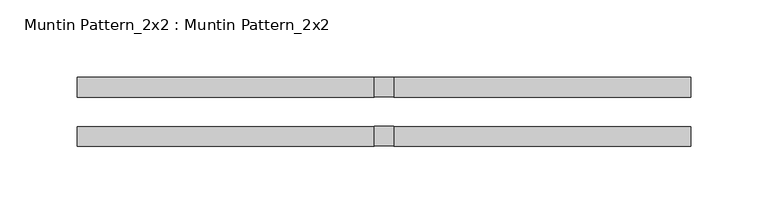
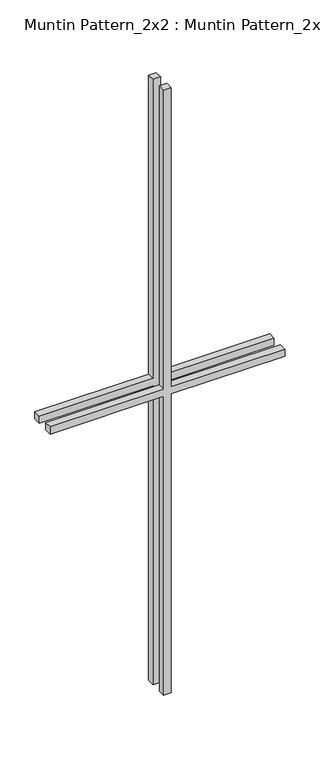
"""IFC4 building model written with IfcOpenShell, lengths in millimetres: proxy geometry, Muntin Pattern_2x2 : Muntin Pattern_2x2."""

from ifc_helpers import new_model, si_unit, frame, origin, place, context, project, spatial, polyline, outline, extrude, source, transform, mapped, element, save


def muntin_pattern_2x2_muntin_pattern_2x2_529c3de1(model_context):
    return source(origin(), model_context, "Body", "SweptSolid", [
        extrude(outline(polyline([(546.1, -6.35), (546.1, -198.4375), (533.4, -198.4375), (533.4, -6.35), (0.0, -6.35), (0.0, 6.35), (533.4, 6.35), (533.4, 198.4375), (546.1, 198.4375), (546.1, 6.35), (1079.5, 6.35), (1079.5, -6.35), (546.1, -6.35)])), frame((0.0, -22.225, 0.0), z_axis=(0.0, 1.0, 0.0), x_axis=(0.0, 0.0, 1.0)), (0.0, 0.0, 1.0), 12.7),
        extrude(outline(polyline([(546.1, -6.35), (546.1, -198.4375), (533.4, -198.4375), (533.4, -6.35), (0.0, -6.35), (0.0, 6.35), (533.4, 6.35), (533.4, 198.4375), (546.1, 198.4375), (546.1, 6.35), (1079.5, 6.35), (1079.5, -6.35), (546.1, -6.35)])), frame((0.0, 9.525, 0.0), z_axis=(0.0, 1.0, 0.0), x_axis=(0.0, 0.0, 1.0)), (0.0, 0.0, 1.0), 12.7),
    ])


if __name__ == "__main__":
    model = new_model("IFC4")
    model_context = context("Model", 3, world=origin())
    ifc_project = project(units=[si_unit("LENGTHUNIT", "METRE", prefix="MILLI")], contexts=[model_context])
    site = spatial("IfcSite", under=ifc_project)
    building = spatial("IfcBuilding", under=site)
    placement = place(None, origin())
    muntin_pattern_2x2_muntin_pattern_2x2_shape = muntin_pattern_2x2_muntin_pattern_2x2_529c3de1(model_context)
    element("IfcBuildingElementProxy", 1, Name="Muntin Pattern_2x2 : Muntin Pattern_2x2", ObjectType="Muntin Pattern_2x2 : Muntin Pattern_2x2", at=placement, inside=building, context=model_context, shape_type="MappedRepresentation", body=[
        mapped(muntin_pattern_2x2_muntin_pattern_2x2_shape, transform((0.0, 0.0, 0.0), x_axis=(1.0, 0.0, 0.0), y_axis=(0.0, 1.0, 0.0), z_axis=(0.0, 0.0, 1.0))),
    ])
    save(model, "model.ifc")

# Revit data of these elements
# Type "Muntin Pattern_2x2 : Muntin Pattern_2x2"
#   Width [instance default] = 4' - 0"
#   Thickness = 0' - 0 1/2"
#   Height [instance default] = 4' - 0"
#   Distance = 0' - 0 3/4"
#   Interior Material [instance default] = none
#   Exterior Material [instance default] = none
#   Default Elevation = 0
# Element 1 (IfcBuildingElementProxy, "Muntin Pattern_2x2 : Muntin Pattern_2x2")
#   Width = 1' - 3 5/8"
#   Height = 3' - 6 1/2"
#   Interior Material = Wood - Stained
#   Exterior Material = Clad - White
#   Materials on its faces: "Clad - White", "Wood - Stained"
# Materials
#   "Clad - White": class "Wood", colour RGB 242 242 238, transparency 0, Cost = 0
#   "Wood - Stained": class "Wood", colour RGB 224 178 126, transparency 0, Cost = 0
